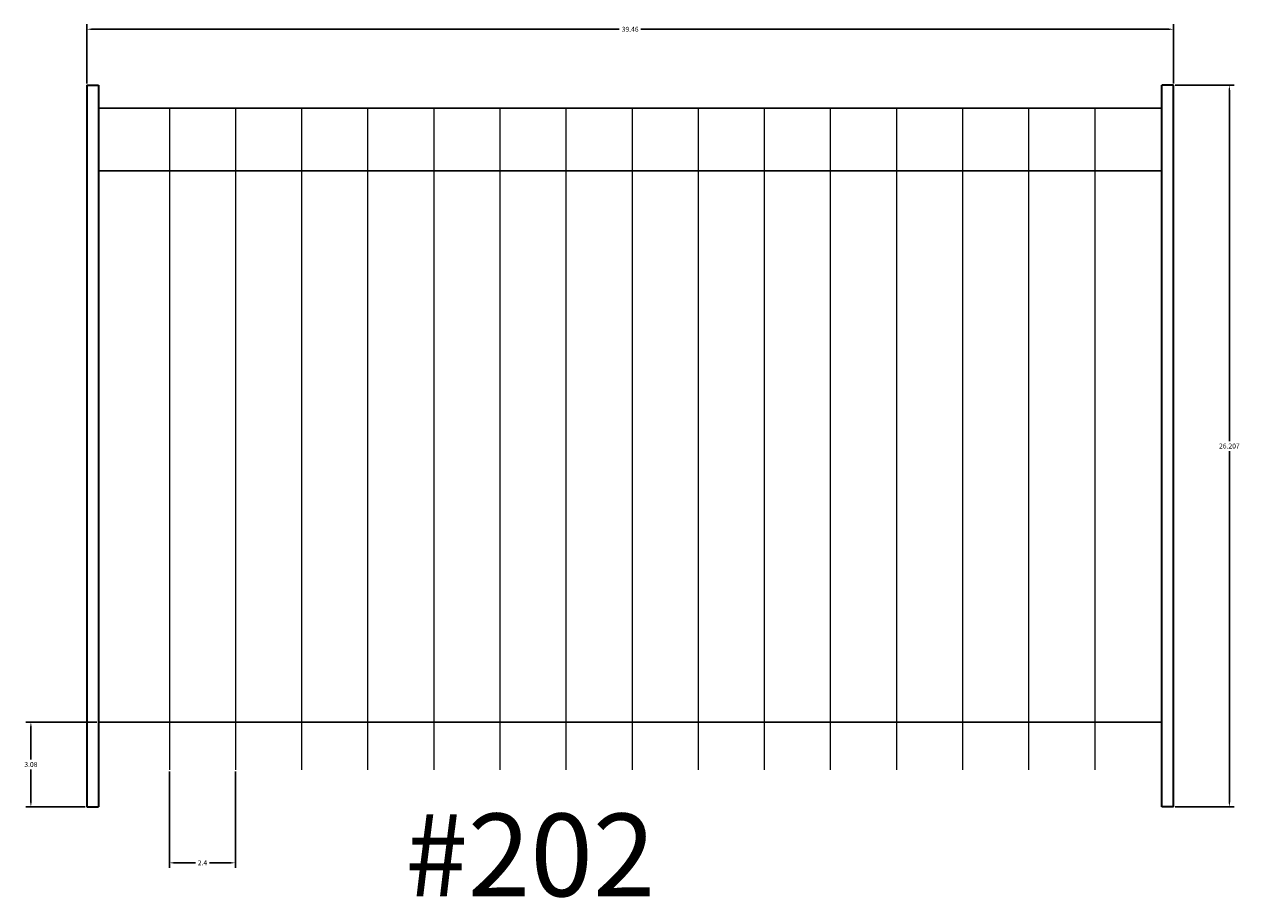
# Model space of a CAD drawing. Units: inches. Extents: x 756 to 915, y 488 to 695.
# Tile 19 of 25: x 815 to 859, y 626 to 658. Entities that reach past the tile are written whole.
import ezdxf

# ---------------------------------------------------------------- set-up
doc = ezdxf.new("R2010")
doc.units = ezdxf.units.IN
doc.header["$MEASUREMENT"] = 0
for name, color, linetype, lineweight in [('L-ANNO-TEXT', 7, 'Continuous', 25), ('L-FENC-PCKT', 7, 'Continuous', 18), ('L-FENC-POST', 7, 'Continuous', 35), ('L-FENC-RAIL', 7, 'Continuous', 25), ('M-DIMS', 2, 'Continuous', 18)]:
    doc.layers.add(name, color=color, linetype=linetype, lineweight=lineweight)
doc.styles.get("Standard").update_dxf_attribs({"font": 'arial.ttf'})
doc.dimstyles.get("Standard").update_dxf_attribs({"dimtxt": 0.18, "dimasz": 0.18, "dimexe": 0.18, "dimexo": 0.0625, "dimgap": 0.09, "dimtad": 0, "dimtih": 1, "dimtoh": 1, "dimdec": 0, "dimzin": 0, "dimdsep": 46, "dimlunit": 3, "dimtxsty": 'Standard', "dimcen": 0.09, "dimadec": 0, "dimazin": 0, "dimtfac": 1, "dimtdec": 0, "dimtofl": 0, "dimtmove": 0, "dimatfit": 3, "dimfxl": 1, "dimtolj": 1, "dimtzin": 0, "dimarcsym": 0})

# ---------------------------------------------------------------- blocks, each defined once
blk = doc.blocks.new('FENCE-POST-LEFT')
for p, q in [((0, 26.207), (0, 0)), ((0, 26.207), (0.426, 26.207)), ((0.426, 26.207), (0.426, 0)), ((0.426, 26.207), (0.426, 0)), ((0, 0), (0.426, 0))]:
    blk.add_line(p, q)
blk = doc.blocks.new('FENCE-POST-RIGHT')
for p, q in [((0, 26.207), (0, 0)), ((0, 26.207), (0.427, 26.207)), ((0.427, 26.207), (0.427, 0)), ((0, 0), (0.427, 0))]:
    blk.add_line(p, q)
blk = doc.blocks.new('*D37')
at = {"layer": 'Defpoints', "color": 0, "transparency": 16777216}
for p in [(856.791, 657.541), (817.333, 655.511), (856.791, 655.511)]:
    blk.add_point(p, dxfattribs=at)
at = {"layer": 'M-DIMS', "color": 0, "lineweight": -2, "transparency": 16777216}
for p, q in [((817.333, 655.574), (817.333, 657.721)), ((856.791, 655.574), (856.791, 657.721)), ((817.513, 657.541), (836.668, 657.541)), ((856.611, 657.541), (837.455, 657.541))]:
    blk.add_line(p, q, dxfattribs=at)
at = {"layer": 'M-DIMS', "color": 0, "transparency": 16777216}
for points in [[(817.513, 657.571), (817.513, 657.511), (817.333, 657.541)], [(856.611, 657.571), (856.611, 657.511), (856.791, 657.541)]]:
    blk.add_solid(points, dxfattribs=at)
at = {"layer": 'M-DIMS', "color": 0, "transparency": 16777216, "insert": (837.062, 657.541), "char_height": 0.18, "attachment_point": 5}
blk.add_mtext('\\A1;39.46', dxfattribs=at)
blk = doc.blocks.new('*D38')
at = {"layer": 'Defpoints', "color": 0, "transparency": 16777216}
for p in [(856.791, 655.511), (858.821, 655.511), (856.791, 629.304)]:
    blk.add_point(p, dxfattribs=at)
at = {"layer": 'M-DIMS', "color": 0, "lineweight": -2, "transparency": 16777216}
for p, q in [((856.853, 655.511), (859.001, 655.511)), ((858.821, 655.331), (858.821, 642.59)), ((858.821, 629.484), (858.821, 642.226)), ((856.853, 629.304), (859.001, 629.304))]:
    blk.add_line(p, q, dxfattribs=at)
at = {"layer": 'M-DIMS', "color": 0, "transparency": 16777216}
for points in [[(858.791, 655.331), (858.851, 655.331), (858.821, 655.511)], [(858.791, 629.484), (858.851, 629.484), (858.821, 629.304)]]:
    blk.add_solid(points, dxfattribs=at)
at = {"layer": 'M-DIMS', "color": 0, "transparency": 16777216, "insert": (858.821, 642.408), "char_height": 0.18, "attachment_point": 5}
blk.add_mtext('\\A1;26.207', dxfattribs=at)
blk = doc.blocks.new('*D39')
at = {"layer": 'Defpoints', "color": 0, "transparency": 16777216}
for p in [(820.332, 630.654), (822.732, 630.654), (822.732, 627.274)]:
    blk.add_point(p, dxfattribs=at)
at = {"layer": 'M-DIMS', "color": 0, "lineweight": -2, "transparency": 16777216}
for p, q in [((820.332, 630.591), (820.332, 627.094)), ((822.732, 630.591), (822.732, 627.094)), ((820.512, 627.274), (821.277, 627.274)), ((822.552, 627.274), (821.787, 627.274))]:
    blk.add_line(p, q, dxfattribs=at)
at = {"layer": 'M-DIMS', "color": 0, "transparency": 16777216}
for points in [[(820.512, 627.304), (820.512, 627.244), (820.332, 627.274)], [(822.552, 627.304), (822.552, 627.244), (822.732, 627.274)]]:
    blk.add_solid(points, dxfattribs=at)
at = {"layer": 'M-DIMS', "color": 0, "transparency": 16777216, "insert": (821.532, 627.274), "char_height": 0.18, "attachment_point": 5}
blk.add_mtext('\\A1;2.4', dxfattribs=at)
blk = doc.blocks.new('*D40')
at = {"layer": 'Defpoints', "color": 0, "transparency": 16777216}
for p in [(815.303, 632.386), (817.759, 632.386), (817.333, 629.304)]:
    blk.add_point(p, dxfattribs=at)
at = {"layer": 'M-DIMS', "color": 0, "lineweight": -2, "transparency": 16777216}
for p, q in [((817.697, 632.386), (815.123, 632.386)), ((815.303, 632.206), (815.303, 631.027)), ((815.303, 629.484), (815.303, 630.663)), ((817.27, 629.304), (815.123, 629.304))]:
    blk.add_line(p, q, dxfattribs=at)
at = {"layer": 'M-DIMS', "color": 0, "transparency": 16777216}
for points in [[(815.273, 632.206), (815.333, 632.206), (815.303, 632.386)], [(815.273, 629.484), (815.333, 629.484), (815.303, 629.304)]]:
    blk.add_solid(points, dxfattribs=at)
at = {"layer": 'M-DIMS', "color": 0, "transparency": 16777216, "insert": (815.303, 630.845), "char_height": 0.18, "attachment_point": 5}
blk.add_mtext('\\A1;3.08', dxfattribs=at)

msp = doc.modelspace()

# ---------------------------------------------------------------- linework, layer by layer
at = {"layer": 'L-FENC-PCKT'}
for p, q in [((820.3317, 654.6726), (820.3317, 630.6539)), ((822.7316, 654.6726), (822.7316, 630.6539)), ((825.1315, 654.6726), (825.1315, 630.6539)), ((827.5314, 654.6726), (827.5314, 630.6539)), ((829.9313, 654.6726), (829.9313, 630.6539)), ((832.3313, 654.6726), (832.3313, 630.6539)), ((834.7312, 654.6726), (834.7312, 630.6539)), ((837.1311, 654.6726), (837.1311, 630.6539)), ((839.531, 654.6726), (839.531, 630.6539)), ((841.9309, 654.6726), (841.9309, 630.6539)), ((844.3308, 654.6726), (844.3308, 630.6539)), ((846.7307, 654.6726), (846.7307, 630.6539)), ((849.1306, 654.6726), (849.1306, 630.6539)), ((851.5305, 654.6726), (851.5305, 630.6539)), ((853.9305, 654.6726), (853.9305, 630.6539))]:
    msp.add_line(p, q, dxfattribs=at)
at = {"layer": 'L-FENC-RAIL'}
for p, q in [((817.7592, 654.6726), (856.3641, 654.6726)), ((817.7592, 652.3962), (856.3641, 652.3962)), ((817.7592, 632.386), (856.3641, 632.386))]:
    msp.add_line(p, q, dxfattribs=at)

# ---------------------------------------------------------------- block references
at = {"layer": 'L-FENC-POST'}
msp.add_blockref('FENCE-POST-LEFT', (817.3329, 629.3043), dxfattribs=at)
at = {"layer": 'L-FENC-POST', "rotation": 180}
msp.add_blockref('FENCE-POST-RIGHT', (856.7909, 655.5112), dxfattribs=at)

# ---------------------------------------------------------------- texts
at = {"layer": 'L-ANNO-TEXT'}
msp.add_text('#202', height=3, dxfattribs=at).set_placement((828.8948, 626.0614))

# ---------------------------------------------------------------- dimensions: what is measured, and where the dimension line sits
at = {"layer": 'M-DIMS'}
for base, p1, p2, override, picture, middle in [((856.7907, 657.5412), (817.3326, 655.5112), (856.7907, 655.5112), {"dimdec": 2, "dimlfac": 1, "dimrnd": 0, "dimzin": 0, "dimdsep": 46, "dimlunit": 2}, '*D37', (837.0617, 657.5412)), ((822.7316, 627.2744), (820.3317, 630.6539), (822.7316, 630.6539), {"dimdec": 1, "dimlfac": 1, "dimrnd": 0, "dimzin": 0, "dimdsep": 46, "dimlunit": 2}, '*D39', (821.5317, 627.2744))]:
    dim = msp.add_linear_dim(base=base, p1=p1, p2=p2, dimstyle='Standard', override=override, dxfattribs=at)
    dim.commit()
    dim.dimension.update_dxf_attribs({"geometry": picture, "text_midpoint": middle})
for base, p1, p2, override, picture, middle in [((858.8207, 655.5112), (856.7907, 629.3044), (856.7907, 655.5112), {"dimdec": 3, "dimlfac": 1, "dimrnd": 0, "dimzin": 0, "dimdsep": 46, "dimlunit": 2}, '*D38', (858.8207, 642.4078)), ((815.3026, 632.386), (817.3326, 629.3044), (817.7592, 632.386), {"dimdec": 2, "dimlfac": 1, "dimrnd": 0, "dimzin": 0, "dimdsep": 46, "dimlunit": 2}, '*D40', (815.3026, 630.8452))]:
    dim = msp.add_linear_dim(base=base, p1=p1, p2=p2, angle=90, dimstyle='Standard', override=override, dxfattribs=at)
    dim.commit()
    dim.dimension.update_dxf_attribs({"geometry": picture, "text_midpoint": middle})

doc.saveas('drawing.dxf')
